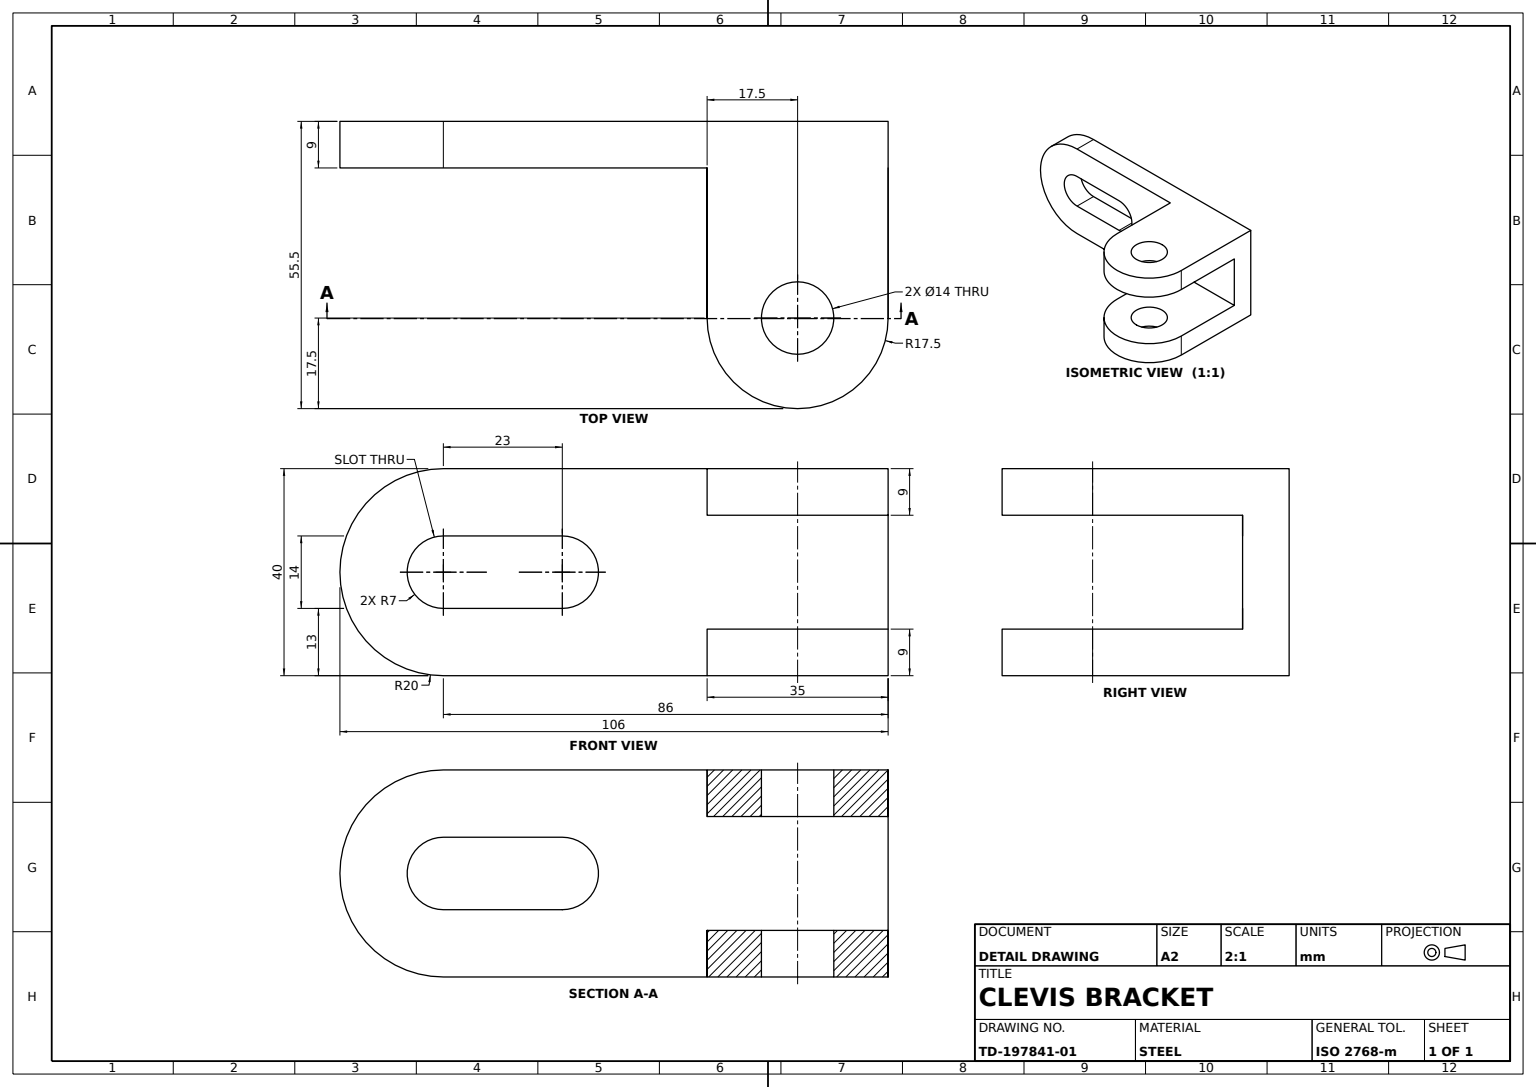
from build123d import *

# Parameters (mm, degrees)
BASE_PLATE_DEPTH   = 9
BASE_SLOT_DEPTH    = 28
CLEVIS_EAR_1_DEPTH = 9
CLEVIS_START       = -9
CLEVIS_EAR_2_DEPTH = 9
PIN_HOLE_SKETCH_R  = 7
PIN_HOLE_DEPTH     = 80


with BuildPart() as part:
    # Base Plate Sketch → Base Plate (new body)
    with BuildSketch(Plane(origin=(0, 0, 0), x_dir=(-1, 0, 0), z_dir=(0, 0, 1))):
        with BuildLine():
            Line((0, 0), (86, 0))
            ThreePointArc((86, 0), (106, 20), (86, 40))
            Line((86, 40), (0, 40))
            Line((0, 40), (0, 0))
        make_face()
    extrude(amount=BASE_PLATE_DEPTH)

    # Base Slot Sketch → Base Slot (cut)
    with BuildSketch(Plane(origin=(0, 0, 0), x_dir=(1, 0, 0), z_dir=(0, 0, -1))):
        with BuildLine():
            Line((-86, 27), (-63, 27))
            ThreePointArc((-63, 27), (-56, 20), (-63, 13))
            Line((-63, 13), (-86, 13))
            ThreePointArc((-86, 13), (-93, 20), (-86, 27))
        make_face()
    extrude(amount=-BASE_SLOT_DEPTH, mode=Mode.SUBTRACT)

    # Clevis Ear 1 Sketch → Clevis Ear 1 (add)
    with BuildSketch(Plane.XZ.offset(40)):
        with BuildLine():
            Line((0, 9), (0, 38))
            ThreePointArc((0, 38), (-17.5, 55.5), (-35, 38))
            Line((-35, 38), (-35, 9))
            Line((-35, 9), (0, 9))
        make_face()
    extrude(amount=-CLEVIS_EAR_1_DEPTH)

    # Clevis Ear 2 Sketch → Clevis Ear 2 (add)
    with BuildSketch(Plane(origin=(0, 0, 0), x_dir=(-1, 0, 0), z_dir=(0, 1, 0)).offset(CLEVIS_START)):
        with BuildLine():
            Line((0, 9), (0, 38))
            ThreePointArc((0, 38), (17.5, 55.5), (35, 38))
            Line((35, 38), (35, 9))
            Line((35, 9), (0, 9))
        make_face()
    extrude(amount=CLEVIS_EAR_2_DEPTH)

    # Pin Hole Sketch → Pin Hole (cut)
    with BuildSketch(Plane(origin=(0, 0, 0), x_dir=(-1, 0, 0), z_dir=(0, 1, 0))):
        with Locations(Location((17.5, 38, 0), (0, 0, 90))):
            Circle(PIN_HOLE_SKETCH_R)
    extrude(amount=-PIN_HOLE_DEPTH, mode=Mode.SUBTRACT)


solid = part.part
